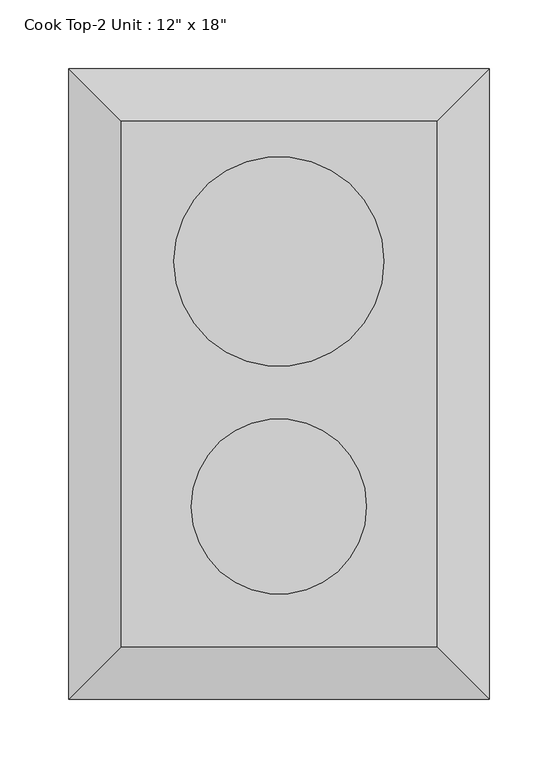
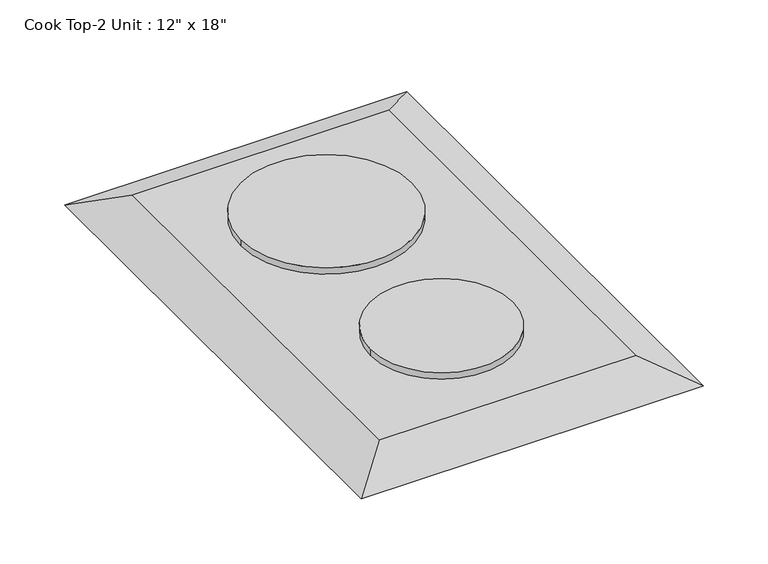
"""IFC4 building model written with IfcOpenShell, lengths in millimetres: proxy geometry."""

from ifc_helpers import new_model, si_unit, point, frame, frame_2d, origin, place, context, project, spatial, circle_curve, trimmed, segment, composite_curve, outline, extrude, faceted_brep, source, transform, mapped, element, save


def proxy_fb8a77b2(model_context):
    return source(origin(), model_context, "Body", "SolidModel", [
        faceted_brep([(190.5, 220.7247956, 933.45), (-38.1, 220.7247956, 933.45), (-38.1, -160.2752044, 933.45), (190.5, -160.2752044, 933.45), (228.6, 258.8247956, 914.4), (228.6, -198.3752044, 914.4), (-76.2, -198.3752044, 914.4), (-76.2, 258.8247956, 914.4)], [[[0, 1, 2, 3]], [[4, 5, 6, 7]], [[4, 7, 1, 0]], [[7, 6, 2, 1]], [[6, 5, 3, 2]], [[5, 4, 0, 3]]]),
        extrude(outline(composite_curve([segment(trimmed(circle_curve(frame_2d((76.2, 119.1247956)), 76.2), [point((152.4, 119.1247956))], [point((0.0, 119.1247956))], False, "CARTESIAN"), True, "CONTINUOUS"), segment(trimmed(circle_curve(frame_2d((76.2, 119.1247956)), 76.2), [point((0.0, 119.1247956))], [point((152.4, 119.1247956))], False, "CARTESIAN"), True, "CONTINUOUS")], self_intersect=False)), frame((0.0, 0.0, 933.45), z_axis=(0.0, 0.0, 1.0), x_axis=(1.0, 0.0, 0.0)), (0.0, 0.0, 1.0), 6.35),
        extrude(outline(composite_curve([segment(trimmed(circle_curve(frame_2d((76.2, -58.6752044)), 63.5), [point((139.7, -58.6752044))], [point((12.7, -58.6752044))], False, "CARTESIAN"), True, "CONTINUOUS"), segment(trimmed(circle_curve(frame_2d((76.2, -58.6752044)), 63.5), [point((12.7, -58.6752044))], [point((139.7, -58.6752044))], False, "CARTESIAN"), True, "CONTINUOUS")], self_intersect=False)), frame((0.0, 0.0, 933.45), z_axis=(0.0, 0.0, 1.0), x_axis=(1.0, 0.0, 0.0)), (0.0, 0.0, 1.0), 6.35),
    ])


if __name__ == "__main__":
    model = new_model("IFC4")
    model_context = context("Model", 3, world=origin())
    ifc_project = project(units=[si_unit("LENGTHUNIT", "METRE", prefix="MILLI")], contexts=[model_context])
    site = spatial("IfcSite", under=ifc_project)
    building = spatial("IfcBuilding", under=site)
    placement = place(None, origin())
    proxy_shape = proxy_fb8a77b2(model_context)
    element("IfcBuildingElementProxy", 1, Name="Cook Top-2 Unit : 12\" x 18\"", ObjectType="Cook Top-2 Unit : 12\" x 18\"", at=placement, inside=building, context=model_context, shape_type="MappedRepresentation", body=[
        mapped(proxy_shape, transform((0.0, 0.0, 0.0), x_axis=(1.0, 0.0, 0.0), y_axis=(0.0, 1.0, 0.0), z_axis=(0.0, 0.0, 1.0))),
    ])
    save(model, "model.ifc")

# Revit data of these elements
# Type "Cook Top-2 Unit : 12\" x 18\""
#   Assembly Code = "E1090400"
#   Counter Height = 3' - 0"
#   Depth = 1' - 6"
#   Width = 1' - 0"
#   Burner Material = Metal - Chrome
#   Cooktop Material = Metal - Steel, Polished
#   Default Elevation = 0
# Element 1 (IfcBuildingElementProxy, "Cook Top-2 Unit : 12\" x 18\"")
#   Materials on its faces: "Metal - Steel, Polished", "Metal - Chrome"
# Materials
#   "Metal - Chrome": class "Metal", colour RGB 247 247 247, transparency 0
#   "Metal - Steel, Polished": colour RGB 57 57 57, transparency 0
